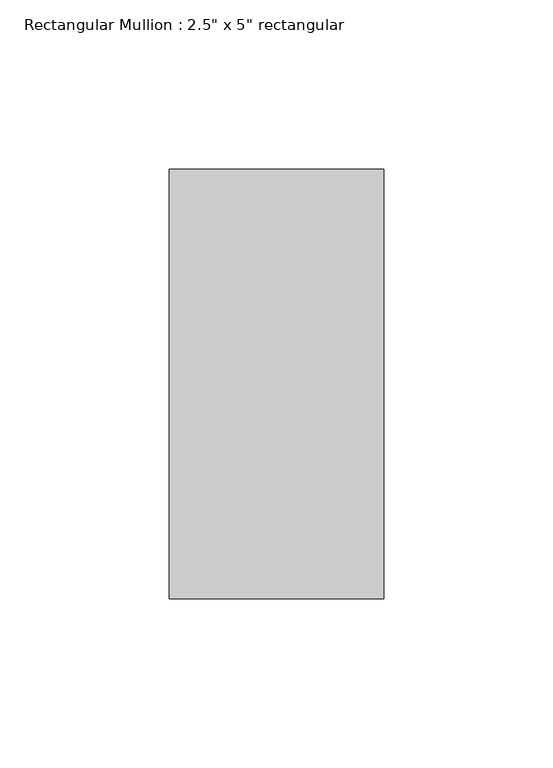
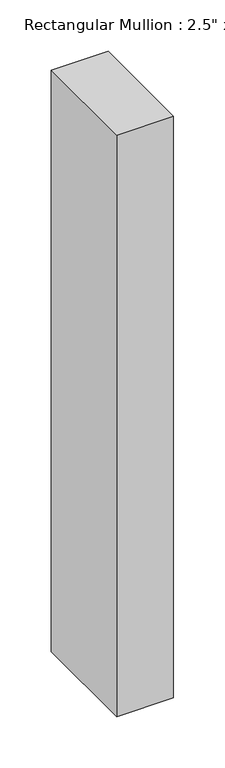
"""IFC4 building model written with IfcOpenShell, lengths in millimetres: member geometry."""

from ifc_helpers import new_model, si_unit, frame, origin, place, context, project, spatial, polyline, outline, extrude, source, transform, mapped, element, save


def member_a2013922(model_context):
    return source(origin(), model_context, "Body", "SweptSolid", [
        extrude(outline(polyline([(0.0, 63.5), (0.0, -63.5), (-63.5, -63.5), (-63.5, 63.5), (0.0, 63.5)])), frame((0.0, 0.0, -689.6941631), z_axis=(0.0, 0.0, 1.0), x_axis=(1.0, 0.0, 0.0)), (0.0, 0.0, 1.0), 689.6941631),
    ])


if __name__ == "__main__":
    model = new_model("IFC4")
    model_context = context("Model", 3, world=origin())
    ifc_project = project(units=[si_unit("LENGTHUNIT", "METRE", prefix="MILLI")], contexts=[model_context])
    site = spatial("IfcSite", under=ifc_project)
    building = spatial("IfcBuilding", under=site)
    placement = place(None, origin())
    member_shape = member_a2013922(model_context)
    element("IfcMember", 1, ObjectType="Rectangular Mullion : 2.5\" x 5\" rectangular", at=placement, inside=building, context=model_context, shape_type="MappedRepresentation", body=[
        mapped(member_shape, transform((0.0, 0.0, 0.0), x_axis=(1.0, 0.0, 0.0), y_axis=(0.0, 1.0, 0.0), z_axis=(0.0, 0.0, 1.0))),
    ])
    save(model, "model.ifc")

# Revit data of these elements
# Type "Rectangular Mullion : 2.5\" x 5\" rectangular"
#   built-in parameter 1007304 = 0.416667 (stored number, unit not read)
#   built-in parameter 1007301 = 0.104167 (stored number, unit not read)
#   built-in parameter 1007300 = 0.104167 (stored number, unit not read)
# Element 1 (IfcMember, "Rectangular Mullion : 2.5\" x 5\" rectangular")
#   Materials on its faces: "Aluminum"
# Materials
#   "Aluminum": class "Metal", colour RGB 247 247 247, transparency 0, Description = "Aluminum 6061", Cost = 0
